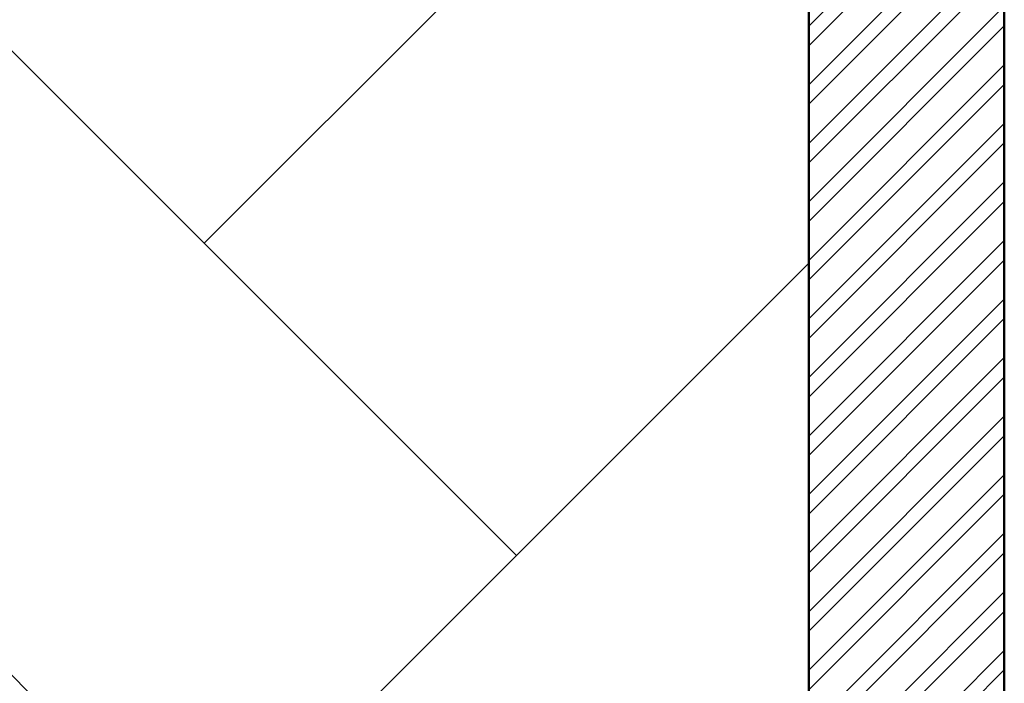
# Model space of a CAD drawing. Units: inches. Extents: x 3590 to 5167, y 65 to 1917.
# Tile 45 of 100: x 5035 to 5080, y 1388 to 1418. Entities that reach past the tile are written whole.
import ezdxf

# ---------------------------------------------------------------- set-up
doc = ezdxf.new("R2010")
doc.units = ezdxf.units.IN
for name, color, linetype, lineweight in [('A-FLOR-PATT', 8, 'Continuous', 13), ('A-WALL', 7, 'Continuous', 50), ('A-WALL-PATT', 251, 'Continuous', 13)]:
    doc.layers.add(name, color=color, linetype=linetype, lineweight=lineweight)

msp = doc.modelspace()

# ---------------------------------------------------------------- hatches: boundary and pattern name
at = {"layer": 'A-FLOR-PATT', "transparency": 33554687}
h = msp.add_hatch(dxfattribs=at)
h.set_pattern_fill('AR-HBONE', color=256, scale=0.2)
h.set_pattern_definition([(45, (-588.972, 0), (0, 28.73682), [60.96, -20.32]), (135, (-574.604, 14.368), (3e-15, 28.73682), [60.96, -20.32])])
h.paths.add_polyline_path([(5071.274, 1796.999), (4933.274, 1796.999), (4933.274, 1753.999), (4962.774, 1753.999, -0.414214), (4928.774, 1719.999), (4933.274, 1718.999), (4933.274, 1334.999), (5071.274, 1334.999)])
h.paths.add_polyline_path([(4951.78, 1521.077), (4951.715, 1521.04), (4951.563, 1520.895)], flags=16)
h.paths.add_polyline_path([(4952.267, 1521.376), (4952.198, 1521.371), (4952.198, 1521.356)], flags=0)
h.paths.add_polyline_path([(4967.051, 1529.728), (4965.231, 1528.694), (4963.411, 1527.714), (4961.756, 1526.851), (4963.589, 1527.449), (4964.036, 1527.478), (4962.975, 1527.249), (4961.76, 1526.852), (4959.792, 1525.834), (4958.005, 1524.895), (4956.24, 1523.93), (4954.504, 1522.919), (4954.129, 1522.682), (4953.361, 1521.997), (4953.366, 1521.998), (4953.605, 1522.064), (4955.106, 1522.761), (4956.921, 1523.434), (4958.678, 1523.915), (4960.358, 1524.2), (4961.945, 1524.286), (4964.171, 1524.108), (4965.958, 1523.309), (4963.863, 1522.976), (4965.187, 1522.499), (4963.366, 1522.497), (4961.545, 1522.487), (4959.764, 1522.461), (4958.304, 1522.419), (4957.974, 1522.388), (4956.307, 1522.232), (4954.718, 1522.071), (4953.251, 1521.899), (4953.525, 1521.623), (4954.331, 1521.379), (4956.243, 1521.23), (4958.039, 1520.93), (4959.684, 1520.483), (4961.16, 1519.896), (4963.107, 1518.8), (4964.393, 1517.325), (4962.973, 1517.726), (4964.558, 1516.661), (4965.407, 1515.708), (4963.507, 1516.322), (4961.68, 1517.005), (4959.935, 1517.745), (4958.282, 1518.528), (4956.732, 1519.343), (4955.295, 1520.175), (4954.672, 1520.572), (4954.513, 1520.627), (4955.658, 1519.318), (4956.703, 1517.982), (4957.644, 1516.647), (4958.485, 1515.334), (4959.55, 1513.524), (4960.438, 1511.769), (4958.841, 1513.62), (4957.452, 1515.325), (4955.819, 1517.459), (4956.665, 1515.448), (4957.111, 1513.923), (4957.447, 1511.714), (4957.076, 1509.793), (4956.538, 1511.11), (4955.992, 1512.569), (4955.444, 1514.125), (4954.898, 1515.735), (4954.357, 1517.356), (4953.824, 1518.943), (4953.305, 1520.452), (4953.065, 1521.116), (4952.971, 1521.146), (4952.949, 1521.086), (4952.73, 1520.199), (4953.37, 1518.024), (4953.757, 1516.373), (4954.051, 1514.765), (4954.264, 1513.221), (4954.471, 1511.131), (4954.497, 1510.402), (4954.409, 1511.76), (4954.264, 1513.221), (4954.051, 1514.765), (4953.757, 1516.373), (4953.37, 1518.024), (4952.877, 1519.698), (4952.716, 1520.141), (4952.533, 1519.059), (4952.374, 1517.789), (4952.219, 1516.312), (4952.046, 1514.6), (4951.833, 1512.626), (4951.557, 1510.363), (4951.203, 1512.168), (4950.852, 1514.339), (4950.985, 1516.376), (4951.66, 1518.286), (4952.593, 1520.481), (4952.357, 1521.13), (4951.855, 1520.328), (4950.839, 1518.908), (4949.777, 1517.587), (4948.916, 1516.617), (4948.111, 1515.256), (4947.089, 1513.554), (4945.889, 1511.615), (4946.326, 1513.402), (4946.562, 1514.249), (4945.528, 1513.327), (4944.581, 1512.531), (4946.018, 1514.508), (4947.204, 1516.048), (4947.893, 1517.313), (4949.307, 1518.764), (4950.414, 1519.767), (4950.451, 1519.806), (4952.267, 1521.376), (4951.645, 1521.493), (4950.404, 1521.18), (4948.044, 1520.359), (4946.119, 1519.452), (4944.572, 1518.475), (4943.35, 1517.443), (4941.997, 1515.92), (4941.661, 1515.275), (4942.813, 1516.99), (4944.572, 1518.475), (4946.119, 1519.452), (4948.044, 1520.359), (4950.404, 1521.18), (4951.645, 1521.493), (4949.647, 1521.868), (4948.6, 1521.756), (4947.126, 1521.57), (4945.42, 1521.348), (4943.45, 1521.105), (4941.183, 1520.856), (4942.86, 1521.613), (4943.873, 1522.03), (4942.952, 1521.909), (4941.41, 1521.485), (4939.543, 1520.67), (4938.968, 1520.226), (4940.733, 1521.299), (4942.952, 1521.909), (4943.702, 1522.008), (4945.894, 1522.7), (4947.565, 1522.714), (4948.921, 1522.566), (4951.131, 1522.183), (4950.971, 1522.297), (4948.129, 1523.006), (4946.035, 1523.707), (4944.232, 1524.521), (4942.707, 1525.461), (4941.444, 1526.537), (4940.43, 1527.761), (4939.649, 1529.143), (4941.421, 1528.122), (4943.147, 1527.132), (4944.841, 1526.175), (4946.514, 1525.25), (4948.179, 1524.359), (4948.365, 1524.263), (4946.475, 1526.045), (4945.181, 1527.54), (4944.19, 1529.033), (4943.496, 1530.54), (4943.278, 1531.36), (4942.498, 1531.919), (4943.114, 1531.762), (4942.959, 1533.659), (4944.14, 1531.989), (4944.612, 1531.323), (4946.202, 1530.463), (4947.486, 1529.509), (4948.79, 1528.226), (4950.368, 1526.237), (4949.485, 1528.155), (4948.851, 1530.123), (4948.491, 1532.041), (4948.381, 1533.918), (4948.501, 1535.76), (4948.827, 1537.573), (4949.418, 1535.565), (4949.957, 1533.569), (4950.464, 1531.586), (4950.961, 1529.617), (4951.391, 1527.954), (4951.724, 1530.687), (4952.201, 1532.58), (4952.889, 1534.33), (4953.77, 1535.951), (4954.827, 1537.46), (4954.521, 1535.39), (4954.273, 1533.937), (4955.58, 1535.663), (4956.748, 1536.739), (4956.159, 1534.78), (4955.589, 1532.873), (4955.043, 1531.006), (4954.525, 1529.166), (4954.038, 1527.341), (4953.638, 1525.733), (4953.611, 1525.586), (4953.398, 1524.166), (4953.382, 1524.009), (4954.07, 1525.476), (4954.912, 1527.022), (4956.136, 1528.894), (4957.847, 1530.577), (4959.376, 1531.54), (4958.256, 1530.104), (4957.143, 1528.663), (4956.066, 1527.243), (4955.056, 1525.871), (4954.141, 1524.571), (4953.352, 1523.372), (4953.311, 1523.303), (4953.273, 1522.925), (4953.261, 1522.382), (4954.103, 1523.373), (4954.63, 1524.284), (4955.961, 1526.358), (4957.23, 1528.13), (4958.421, 1529.609), (4960.037, 1531.368), (4961.374, 1532.375), (4962.101, 1532.77), (4961.07, 1531.061), (4959.987, 1529.438), (4958.869, 1527.908), (4958.15, 1527.007), (4959.803, 1528.003), (4961.589, 1528.793), (4963.391, 1529.328), (4965.211, 1529.632)], flags=16)
h.paths.add_polyline_path([(4962.944, 1523.182), (4961.107, 1523.422), (4960.392, 1523.362), (4962.35, 1523.331)], flags=0)
h.paths.add_polyline_path([(5049.541, 1584.551), (5049.476, 1584.515), (5049.325, 1584.37)], flags=16)
h.paths.add_polyline_path([(5050.028, 1584.851), (5049.959, 1584.845), (5049.959, 1584.83)], flags=0)
h.paths.add_polyline_path([(5042.333, 1581.949), (5043.88, 1582.926), (5045.806, 1583.833), (5048.165, 1584.654), (5049.406, 1584.967), (5047.408, 1585.342), (5046.361, 1585.231), (5044.888, 1585.044), (5043.181, 1584.822), (5041.211, 1584.579), (5038.944, 1584.33), (5040.622, 1585.087), (5041.634, 1585.504), (5040.713, 1585.383), (5039.171, 1584.959), (5037.304, 1584.144), (5036.729, 1583.7), (5038.494, 1584.773), (5040.713, 1585.383), (5041.463, 1585.482), (5043.655, 1586.174), (5045.326, 1586.188), (5046.682, 1586.04), (5048.893, 1585.657), (5048.732, 1585.771), (5045.891, 1586.48), (5043.796, 1587.181), (5041.994, 1587.996), (5040.468, 1588.935), (5039.205, 1590.011), (5038.191, 1591.235), (5037.41, 1592.617), (5039.182, 1591.596), (5040.909, 1590.607), (5042.602, 1589.649), (5044.275, 1588.724), (5045.94, 1587.833), (5046.126, 1587.738), (5044.237, 1589.519), (5042.942, 1591.015), (5041.952, 1592.508), (5041.257, 1594.014), (5041.039, 1594.834), (5040.26, 1595.393), (5040.875, 1595.237), (5040.721, 1597.133), (5041.901, 1595.463), (5042.373, 1594.798), (5043.963, 1593.938), (5045.247, 1592.983), (5046.552, 1591.701), (5048.129, 1589.712), (5047.247, 1591.63), (5046.613, 1593.597), (5046.252, 1595.515), (5046.142, 1597.392), (5046.262, 1599.234), (5046.588, 1601.047), (5047.179, 1599.039), (5047.718, 1597.043), (5048.225, 1595.06), (5048.722, 1593.091), (5049.152, 1591.429), (5049.485, 1594.161), (5049.962, 1596.054), (5050.65, 1597.804), (5051.532, 1599.425), (5052.589, 1600.934), (5052.283, 1598.864), (5052.034, 1597.411), (5053.341, 1599.137), (5054.509, 1600.213), (5053.92, 1598.254), (5053.35, 1596.348), (5052.805, 1594.48), (5052.286, 1592.64), (5051.799, 1590.815), (5051.4, 1589.207), (5051.373, 1589.06), (5051.159, 1587.64), (5051.143, 1587.483), (5051.831, 1588.95), (5052.673, 1590.496), (5053.898, 1592.368), (5055.608, 1594.051), (5057.137, 1595.014), (5056.017, 1593.578), (5054.904, 1592.137), (5053.828, 1590.717), (5052.817, 1589.345), (5051.902, 1588.046), (5051.113, 1586.846), (5051.072, 1586.777), (5051.034, 1586.399), (5051.022, 1585.856), (5051.864, 1586.847), (5052.391, 1587.758), (5053.723, 1589.832), (5054.991, 1591.604), (5056.182, 1593.083), (5057.798, 1594.842), (5059.135, 1595.849), (5059.863, 1596.244), (5058.831, 1594.535), (5057.749, 1592.912), (5056.63, 1591.382), (5055.912, 1590.482), (5057.564, 1591.477), (5059.35, 1592.267), (5061.152, 1592.802), (5062.972, 1593.106), (5064.812, 1593.203), (5062.992, 1592.169), (5061.172, 1591.188), (5059.518, 1590.325), (5061.35, 1590.924), (5061.797, 1590.952), (5060.737, 1590.723), (5059.521, 1590.326), (5057.553, 1589.308), (5055.766, 1588.369), (5054.002, 1587.404), (5052.265, 1586.393), (5051.891, 1586.156), (5051.122, 1585.471), (5051.127, 1585.472), (5051.366, 1585.538), (5052.867, 1586.235), (5054.682, 1586.908), (5056.439, 1587.389), (5058.12, 1587.675), (5059.706, 1587.76), (5061.933, 1587.583), (5063.719, 1586.783), (5061.624, 1586.45), (5062.949, 1585.973), (5061.127, 1585.971), (5059.307, 1585.961), (5057.525, 1585.935), (5056.065, 1585.893), (5055.735, 1585.862), (5054.068, 1585.707), (5052.479, 1585.546), (5051.012, 1585.373), (5051.286, 1585.097), (5052.092, 1584.853), (5054.004, 1584.704), (5055.8, 1584.404), (5057.446, 1583.958), (5058.921, 1583.37), (5060.868, 1582.274), (5062.154, 1580.799), (5060.734, 1581.2), (5062.32, 1580.135), (5063.168, 1579.182), (5061.269, 1579.796), (5059.441, 1580.479), (5057.696, 1581.219), (5056.043, 1582.003), (5054.493, 1582.817), (5053.057, 1583.649), (5052.433, 1584.047), (5052.274, 1584.101), (5053.42, 1582.793), (5054.464, 1581.457), (5055.405, 1580.121), (5056.247, 1578.809), (5057.311, 1576.998), (5058.199, 1575.244), (5056.602, 1577.094), (5055.213, 1578.799), (5053.58, 1580.933), (5054.427, 1578.922), (5054.872, 1577.397), (5055.208, 1575.189), (5054.838, 1573.267), (5054.299, 1574.584), (5053.754, 1576.043), (5053.206, 1577.599), (5052.659, 1579.209), (5052.118, 1580.83), (5051.585, 1582.417), (5051.066, 1583.927), (5050.826, 1584.59), (5050.733, 1584.62), (5050.711, 1584.561), (5050.491, 1583.673), (5051.131, 1581.498), (5051.518, 1579.847), (5051.813, 1578.24), (5052.026, 1576.695), (5052.233, 1574.605), (5052.258, 1573.876), (5052.17, 1575.234), (5052.026, 1576.695), (5051.813, 1578.24), (5051.518, 1579.847), (5051.131, 1581.498), (5050.638, 1583.172), (5050.477, 1583.615), (5050.294, 1582.533), (5050.136, 1581.263), (5049.981, 1579.786), (5049.807, 1578.074), (5049.594, 1576.1), (5049.318, 1573.837), (5048.965, 1575.642), (5048.613, 1577.813), (5048.747, 1579.85), (5049.421, 1581.76), (5050.354, 1583.955), (5050.118, 1584.604), (5049.616, 1583.802), (5048.6, 1582.382), (5047.538, 1581.061), (5046.677, 1580.091), (5045.872, 1578.73), (5044.85, 1577.028), (5043.651, 1575.089), (5044.087, 1576.877), (5044.324, 1577.723), (5043.289, 1576.801), (5042.342, 1576.005), (5043.779, 1577.982), (5044.966, 1579.522), (5045.655, 1580.787), (5047.068, 1582.239), (5048.175, 1583.241), (5048.213, 1583.28), (5050.028, 1584.851), (5049.406, 1584.967), (5048.165, 1584.654), (5045.806, 1583.833), (5043.88, 1582.926), (5042.333, 1581.949), (5041.111, 1580.917), (5039.758, 1579.394), (5039.423, 1578.749), (5040.575, 1580.464)], flags=16)
h.paths.add_polyline_path([(4954.799, 1533.12), (4954.262, 1532.079), (4953.831, 1530.935), (4953.505, 1529.636), (4953.283, 1528.133), (4953.167, 1526.376), (4953.156, 1524.315), (4953.277, 1521.236), (4952.802, 1521.842), (4951.557, 1521.998), (4950.976, 1521.961), (4952.661, 1521.941), (4952.802, 1521.842), (4953.152, 1523.593), (4953.167, 1526.376), (4953.283, 1528.133), (4953.609, 1530.346), (4954.456, 1532.592)], flags=0)
h.paths.add_polyline_path([(5050.563, 1585.316), (5049.318, 1585.472), (5048.737, 1585.435), (5050.422, 1585.415), (5050.563, 1585.316), (5050.914, 1587.067), (5050.928, 1589.851), (5051.045, 1591.607), (5051.371, 1593.82), (5052.217, 1596.066), (5052.56, 1596.594), (5052.024, 1595.554), (5051.592, 1594.409), (5051.266, 1593.11), (5051.045, 1591.607), (5050.928, 1589.851), (5050.918, 1587.789), (5051.038, 1584.71)], flags=0)
h.paths.add_polyline_path([(5058.153, 1586.836), (5060.111, 1586.805), (5060.705, 1586.656), (5058.868, 1586.896)], flags=0)
h.paths.add_polyline_path([(5049.541, 1430.936), (5049.476, 1430.9), (5049.325, 1430.755)], flags=16)
h.paths.add_polyline_path([(5050.028, 1431.236), (5049.959, 1431.231), (5049.959, 1431.215)], flags=0)
h.paths.add_polyline_path([(5046.588, 1447.432), (5047.179, 1445.425), (5047.718, 1443.429), (5048.225, 1441.446), (5048.722, 1439.476), (5049.152, 1437.814), (5049.485, 1440.546), (5049.962, 1442.439), (5050.65, 1444.189), (5051.532, 1445.811), (5052.589, 1447.319), (5052.283, 1445.249), (5052.034, 1443.796), (5053.341, 1445.522), (5054.509, 1446.598), (5053.92, 1444.64), (5053.35, 1442.733), (5052.805, 1440.865), (5052.286, 1439.025), (5051.799, 1437.201), (5051.4, 1435.592), (5051.373, 1435.445), (5051.159, 1434.025), (5051.143, 1433.868), (5051.831, 1435.335), (5052.673, 1436.881), (5053.898, 1438.753), (5055.608, 1440.436), (5057.137, 1441.4), (5056.017, 1439.963), (5054.904, 1438.522), (5053.828, 1437.102), (5052.817, 1435.73), (5051.902, 1434.431), (5051.113, 1433.231), (5051.072, 1433.162), (5051.034, 1432.784), (5051.022, 1432.242), (5051.864, 1433.232), (5052.391, 1434.143), (5053.723, 1436.217), (5054.991, 1437.989), (5056.182, 1439.468), (5057.798, 1441.227), (5059.135, 1442.235), (5059.863, 1442.629), (5058.831, 1440.921), (5057.749, 1439.298), (5056.63, 1437.767), (5055.912, 1436.867), (5057.564, 1437.863), (5059.35, 1438.652), (5061.152, 1439.187), (5062.972, 1439.491), (5064.812, 1439.588), (5062.992, 1438.554), (5061.172, 1437.573), (5059.518, 1436.71), (5061.35, 1437.309), (5061.797, 1437.337), (5060.737, 1437.108), (5059.521, 1436.711), (5057.553, 1435.693), (5055.766, 1434.754), (5054.002, 1433.789), (5052.265, 1432.778), (5051.891, 1432.541), (5051.122, 1431.856), (5051.127, 1431.857), (5051.366, 1431.923), (5052.867, 1432.62), (5054.682, 1433.293), (5056.439, 1433.775), (5058.12, 1434.06), (5059.706, 1434.145), (5061.933, 1433.968), (5063.719, 1433.168), (5061.624, 1432.835), (5062.949, 1432.358), (5061.127, 1432.357), (5059.307, 1432.346), (5057.525, 1432.32), (5056.065, 1432.278), (5055.735, 1432.248), (5054.068, 1432.092), (5052.479, 1431.931), (5051.012, 1431.759), (5051.286, 1431.482), (5052.092, 1431.238), (5054.004, 1431.089), (5055.8, 1430.789), (5057.446, 1430.343), (5058.921, 1429.755), (5060.868, 1428.66), (5062.154, 1427.185), (5060.734, 1427.585), (5062.32, 1426.52), (5063.168, 1425.567), (5061.269, 1426.181), (5059.441, 1426.865), (5057.696, 1427.604), (5056.043, 1428.388), (5054.493, 1429.202), (5053.057, 1430.034), (5052.433, 1430.432), (5052.274, 1430.487), (5053.42, 1429.178), (5054.464, 1427.842), (5055.405, 1426.506), (5056.247, 1425.194), (5057.311, 1423.383), (5058.199, 1421.629), (5056.602, 1423.479), (5055.213, 1425.184), (5053.58, 1427.318), (5054.427, 1425.307), (5054.872, 1423.782), (5055.208, 1421.574), (5054.838, 1419.652), (5054.299, 1420.97), (5053.754, 1422.428), (5053.206, 1423.984), (5052.659, 1425.595), (5052.118, 1427.215), (5051.585, 1428.802), (5051.066, 1430.312), (5050.826, 1430.975), (5050.733, 1431.005), (5050.711, 1430.946), (5050.491, 1430.058), (5051.131, 1427.883), (5051.518, 1426.232), (5051.813, 1424.625), (5052.026, 1423.081), (5052.233, 1420.991), (5052.258, 1420.261), (5052.17, 1421.619), (5052.026, 1423.081), (5051.813, 1424.625), (5051.518, 1426.232), (5051.131, 1427.883), (5050.638, 1429.558), (5050.477, 1430.001), (5050.294, 1428.918), (5050.136, 1427.648), (5049.981, 1426.171), (5049.807, 1424.459), (5049.594, 1422.485), (5049.318, 1420.222), (5048.965, 1422.028), (5048.613, 1424.199), (5048.747, 1426.235), (5049.421, 1428.146), (5050.354, 1430.34), (5050.118, 1430.989), (5049.616, 1430.187), (5048.6, 1428.768), (5047.538, 1427.446), (5046.677, 1426.477), (5045.872, 1425.116), (5044.85, 1423.413), (5043.651, 1421.474), (5044.087, 1423.262), (5044.324, 1424.109), (5043.289, 1423.186), (5042.342, 1422.391), (5043.779, 1424.368), (5044.966, 1425.907), (5045.655, 1427.173), (5047.068, 1428.624), (5048.175, 1429.627), (5048.213, 1429.666), (5050.028, 1431.236), (5049.406, 1431.353), (5048.165, 1431.039), (5045.806, 1430.218), (5043.88, 1429.311), (5042.333, 1428.334), (5041.111, 1427.302), (5039.758, 1425.779), (5039.423, 1425.134), (5040.575, 1426.849), (5042.333, 1428.334), (5043.88, 1429.311), (5045.806, 1430.218), (5048.165, 1431.039), (5049.406, 1431.353), (5047.408, 1431.727), (5046.361, 1431.616), (5044.888, 1431.429), (5043.181, 1431.207), (5041.211, 1430.964), (5038.944, 1430.715), (5040.622, 1431.472), (5041.634, 1431.89), (5040.713, 1431.769), (5039.171, 1431.345), (5037.304, 1430.53), (5036.729, 1430.085), (5038.494, 1431.158), (5040.713, 1431.769), (5041.463, 1431.867), (5043.655, 1432.559), (5045.326, 1432.573), (5046.682, 1432.425), (5048.893, 1432.042), (5048.732, 1432.156), (5045.891, 1432.865), (5043.796, 1433.566), (5041.994, 1434.381), (5040.468, 1435.321), (5039.205, 1436.396), (5038.191, 1437.62), (5037.41, 1439.002), (5039.182, 1437.982), (5040.909, 1436.992), (5042.602, 1436.034), (5044.275, 1435.109), (5045.94, 1434.218), (5046.126, 1434.123), (5044.237, 1435.904), (5042.942, 1437.4), (5041.952, 1438.893), (5041.257, 1440.399), (5041.039, 1441.219), (5040.26, 1441.778), (5040.875, 1441.622), (5040.721, 1443.518), (5041.901, 1441.848), (5042.373, 1441.183), (5043.963, 1440.323), (5045.247, 1439.369), (5046.552, 1438.086), (5048.129, 1436.097), (5047.247, 1438.015), (5046.613, 1439.982), (5046.252, 1441.901), (5046.142, 1443.778), (5046.262, 1445.619)], flags=16)
h.paths.add_polyline_path([(5052.382, 1444.255), (5051.623, 1442.78), (5052.024, 1441.939), (5052.56, 1442.98)], flags=0)
h.paths.add_polyline_path([(5050.563, 1431.701), (5049.318, 1431.857), (5048.737, 1431.821), (5050.422, 1431.8)], flags=0)
h.paths.add_polyline_path([(5058.153, 1433.221), (5060.111, 1433.19), (5060.705, 1433.041), (5058.868, 1433.281)], flags=0)
h.paths.add_polyline_path([(5049.541, 1352.285), (5049.476, 1352.249), (5049.325, 1352.104)], flags=16)
h.paths.add_polyline_path([(5050.028, 1352.585), (5049.959, 1352.58), (5049.959, 1352.564)], flags=0)
h.paths.add_polyline_path([(5046.588, 1368.781), (5047.179, 1366.774), (5047.718, 1364.778), (5048.225, 1362.795), (5048.722, 1360.825), (5049.152, 1359.163), (5049.485, 1361.896), (5049.962, 1363.789), (5050.65, 1365.538), (5051.532, 1367.16), (5052.589, 1368.669), (5052.283, 1366.598), (5052.034, 1365.145), (5053.341, 1366.871), (5054.509, 1367.947), (5053.92, 1365.989), (5053.35, 1364.082), (5052.805, 1362.214), (5052.286, 1360.374), (5051.799, 1358.55), (5051.4, 1356.942), (5051.373, 1356.794), (5051.159, 1355.374), (5051.143, 1355.218), (5051.831, 1356.684), (5052.673, 1358.23), (5053.898, 1360.102), (5055.608, 1361.786), (5057.137, 1362.749), (5056.017, 1361.313), (5054.904, 1359.872), (5053.828, 1358.452), (5052.817, 1357.079), (5051.902, 1355.78), (5051.113, 1354.581), (5051.072, 1354.512), (5051.034, 1354.133), (5051.022, 1353.591), (5051.864, 1354.581), (5052.391, 1355.492), (5053.723, 1357.566), (5054.991, 1359.338), (5056.182, 1360.817), (5057.798, 1362.577), (5059.135, 1363.584), (5059.863, 1363.979), (5058.831, 1362.27), (5057.749, 1360.647), (5056.63, 1359.117), (5055.912, 1358.216), (5057.564, 1359.212), (5059.35, 1360.001), (5061.152, 1360.536), (5062.972, 1360.841), (5064.812, 1360.937), (5062.992, 1359.903), (5061.172, 1358.923), (5059.518, 1358.059), (5061.35, 1358.658), (5061.797, 1358.687), (5060.737, 1358.458), (5059.521, 1358.061), (5057.553, 1357.043), (5055.766, 1356.103), (5054.002, 1355.138), (5052.265, 1354.127), (5051.891, 1353.89), (5051.122, 1353.206), (5051.127, 1353.206), (5051.366, 1353.272), (5052.867, 1353.969), (5054.682, 1354.643), (5056.439, 1355.124), (5058.12, 1355.409), (5059.706, 1355.495), (5061.933, 1355.317), (5063.719, 1354.518), (5061.624, 1354.184), (5062.949, 1353.708), (5061.127, 1353.706), (5059.307, 1353.695), (5057.525, 1353.669), (5056.065, 1353.627), (5055.735, 1353.597), (5054.068, 1353.441), (5052.479, 1353.28), (5051.012, 1353.108), (5051.286, 1352.831), (5052.092, 1352.587), (5054.004, 1352.439), (5055.8, 1352.138), (5057.446, 1351.692), (5058.921, 1351.104), (5060.868, 1350.009), (5062.154, 1348.534), (5060.734, 1348.935), (5062.32, 1347.869), (5063.168, 1346.916), (5061.269, 1347.53), (5059.441, 1348.214), (5057.696, 1348.954), (5056.043, 1349.737), (5054.493, 1350.551), (5053.057, 1351.383), (5052.433, 1351.781), (5052.274, 1351.836), (5053.42, 1350.527), (5054.464, 1349.191), (5055.405, 1347.855), (5056.247, 1346.543), (5057.311, 1344.733), (5058.199, 1342.978), (5056.602, 1344.828), (5055.213, 1346.534), (5053.58, 1348.667), (5054.427, 1346.656), (5054.872, 1345.132), (5055.208, 1342.923), (5054.838, 1341.002), (5054.299, 1342.319), (5053.754, 1343.778), (5053.206, 1345.334), (5052.659, 1346.944), (5052.118, 1348.564), (5051.585, 1350.151), (5051.066, 1351.661), (5050.826, 1352.324), (5050.733, 1352.355), (5050.711, 1352.295), (5050.491, 1351.408), (5051.131, 1349.232), (5051.518, 1347.581), (5051.813, 1345.974), (5052.026, 1344.43), (5052.233, 1342.34), (5052.258, 1341.61), (5052.17, 1342.969), (5052.026, 1344.43), (5051.813, 1345.974), (5051.518, 1347.581), (5051.131, 1349.232), (5050.638, 1350.907), (5050.477, 1351.35), (5050.294, 1350.267), (5050.136, 1348.997), (5049.981, 1347.52), (5049.807, 1345.809), (5049.594, 1343.835), (5049.318, 1341.571), (5048.965, 1343.377), (5048.613, 1345.548), (5048.747, 1347.585), (5049.421, 1349.495), (5050.354, 1351.689), (5050.118, 1352.339), (5049.616, 1351.536), (5048.6, 1350.117), (5047.538, 1348.795), (5046.677, 1347.826), (5045.872, 1346.465), (5044.85, 1344.763), (5043.651, 1342.824), (5044.087, 1344.611), (5044.324, 1345.458), (5043.289, 1344.535), (5042.342, 1343.74), (5043.779, 1345.717), (5044.966, 1347.256), (5045.655, 1348.522), (5047.068, 1349.973), (5048.175, 1350.976), (5048.213, 1351.015), (5050.028, 1352.585), (5049.406, 1352.702), (5048.165, 1352.388), (5045.806, 1351.567), (5043.88, 1350.661), (5042.333, 1349.683), (5041.111, 1348.651), (5039.758, 1347.128), (5039.423, 1346.483), (5040.575, 1348.198), (5042.333, 1349.683), (5043.88, 1350.661), (5045.806, 1351.567), (5048.165, 1352.388), (5049.406, 1352.702), (5047.408, 1353.076), (5046.361, 1352.965), (5044.888, 1352.779), (5043.181, 1352.556), (5041.211, 1352.313), (5038.944, 1352.065), (5040.622, 1352.821), (5041.634, 1353.239), (5040.713, 1353.118), (5039.171, 1352.694), (5037.304, 1351.879), (5036.729, 1351.434), (5038.494, 1352.508), (5040.713, 1353.118), (5041.463, 1353.216), (5043.655, 1353.909), (5045.326, 1353.923), (5046.682, 1353.774), (5048.893, 1353.391), (5048.732, 1353.506), (5045.891, 1354.214), (5043.796, 1354.915), (5041.994, 1355.73), (5040.468, 1356.67), (5039.205, 1357.746), (5038.191, 1358.969), (5037.41, 1360.352), (5039.182, 1359.331), (5040.909, 1358.341), (5042.602, 1357.383), (5044.275, 1356.458), (5045.94, 1355.567), (5046.126, 1355.472), (5044.237, 1357.253), (5042.942, 1358.749), (5041.952, 1360.242), (5041.257, 1361.748), (5041.039, 1362.568), (5040.26, 1363.128), (5040.875, 1362.971), (5040.721, 1364.867), (5041.901, 1363.197), (5042.373, 1362.532), (5043.963, 1361.672), (5045.247, 1360.718), (5046.552, 1359.435), (5048.129, 1357.446), (5047.247, 1359.364), (5046.613, 1361.331), (5046.252, 1363.25), (5046.142, 1365.127), (5046.262, 1366.969)], flags=16)
h.paths.add_polyline_path([(5052.382, 1365.604), (5051.623, 1364.129), (5052.024, 1363.288), (5052.56, 1364.329)], flags=0)
h.paths.add_polyline_path([(4951.78, 1698.041), (4951.715, 1698.005), (4951.563, 1697.859)], flags=16)
h.paths.add_polyline_path([(4952.267, 1698.341), (4952.198, 1698.335), (4952.198, 1698.32)], flags=0)
h.paths.add_polyline_path([(4957.076, 1686.757), (4956.538, 1688.074), (4955.992, 1689.533), (4955.444, 1691.089), (4954.898, 1692.699), (4954.357, 1694.32), (4953.824, 1695.907), (4953.305, 1697.417), (4953.065, 1698.08), (4952.971, 1698.11), (4952.949, 1698.051), (4952.73, 1697.163), (4953.37, 1694.988), (4953.757, 1693.337), (4954.051, 1691.729), (4954.264, 1690.185), (4954.471, 1688.095), (4954.497, 1687.366), (4954.409, 1688.724), (4954.264, 1690.185), (4954.051, 1691.729), (4953.757, 1693.337), (4953.37, 1694.988), (4952.877, 1696.662), (4952.716, 1697.105), (4952.533, 1696.023), (4952.374, 1694.753), (4952.219, 1693.276), (4952.046, 1691.564), (4951.833, 1689.59), (4951.557, 1687.327), (4951.203, 1689.132), (4950.852, 1691.303), (4950.985, 1693.34), (4951.66, 1695.25), (4952.593, 1697.445), (4952.357, 1698.094), (4951.855, 1697.292), (4950.839, 1695.872), (4949.777, 1694.551), (4948.916, 1693.581), (4948.111, 1692.22), (4947.089, 1690.518), (4945.889, 1688.579), (4946.326, 1690.366), (4946.562, 1691.213), (4945.528, 1690.291), (4944.581, 1689.495), (4946.018, 1691.472), (4947.204, 1693.012), (4947.893, 1694.277), (4949.307, 1695.729), (4950.414, 1696.731), (4950.451, 1696.77), (4952.267, 1698.341), (4951.645, 1698.457), (4950.404, 1698.144), (4948.044, 1697.323), (4946.119, 1696.416), (4944.572, 1695.439), (4943.35, 1694.407), (4941.997, 1692.884), (4941.661, 1692.239), (4942.813, 1693.954), (4944.572, 1695.439), (4946.119, 1696.416), (4948.044, 1697.323), (4950.404, 1698.144), (4951.645, 1698.457), (4949.647, 1698.832), (4948.6, 1698.72), (4947.126, 1698.534), (4945.42, 1698.312), (4943.45, 1698.069), (4941.183, 1697.82), (4942.86, 1698.577), (4943.873, 1698.994), (4942.952, 1698.873), (4941.41, 1698.449), (4939.543, 1697.634), (4938.968, 1697.19), (4940.733, 1698.263), (4942.952, 1698.873), (4943.702, 1698.972), (4945.894, 1699.664), (4947.565, 1699.678), (4948.921, 1699.53), (4951.131, 1699.147), (4950.971, 1699.261), (4948.129, 1699.97), (4946.035, 1700.671), (4944.232, 1701.486), (4942.707, 1702.425), (4941.444, 1703.501), (4940.43, 1704.725), (4939.649, 1706.107), (4941.421, 1705.086), (4943.147, 1704.097), (4944.841, 1703.139), (4946.514, 1702.214), (4948.179, 1701.323), (4948.365, 1701.227), (4946.475, 1703.009), (4945.181, 1704.505), (4944.19, 1705.997), (4943.496, 1707.504), (4943.278, 1708.324), (4942.498, 1708.883), (4943.114, 1708.727), (4942.959, 1710.623), (4944.14, 1708.953), (4944.612, 1708.287), (4946.202, 1707.428), (4947.486, 1706.473), (4948.79, 1705.191), (4950.368, 1703.202), (4949.485, 1705.12), (4948.851, 1707.087), (4948.491, 1709.005), (4948.381, 1710.882), (4948.501, 1712.724), (4948.827, 1714.537), (4949.418, 1712.529), (4949.957, 1710.533), (4950.464, 1708.55), (4950.961, 1706.581), (4951.391, 1704.919), (4951.724, 1707.651), (4952.201, 1709.544), (4952.889, 1711.294), (4953.77, 1712.915), (4954.827, 1714.424), (4954.521, 1712.354), (4954.273, 1710.901), (4955.58, 1712.627), (4956.748, 1713.703), (4956.159, 1711.744), (4955.589, 1709.837), (4955.043, 1707.97), (4954.525, 1706.13), (4954.038, 1704.305), (4953.638, 1702.697), (4953.611, 1702.55), (4953.398, 1701.13), (4953.382, 1700.973), (4954.07, 1702.44), (4954.912, 1703.986), (4956.136, 1705.858), (4957.847, 1707.541), (4959.376, 1708.504), (4958.256, 1707.068), (4957.143, 1705.627), (4956.066, 1704.207), (4955.056, 1702.835), (4954.141, 1701.536), (4953.352, 1700.336), (4953.311, 1700.267), (4953.273, 1699.889), (4953.261, 1699.346), (4954.103, 1700.337), (4954.63, 1701.248), (4955.961, 1703.322), (4957.23, 1705.094), (4958.421, 1706.573), (4960.037, 1708.332), (4961.374, 1709.339), (4962.101, 1709.734), (4961.07, 1708.025), (4959.987, 1706.402), (4958.869, 1704.872), (4958.15, 1703.972), (4959.803, 1704.967), (4961.589, 1705.757), (4963.391, 1706.292), (4965.211, 1706.596), (4967.051, 1706.692), (4965.231, 1705.659), (4963.411, 1704.678), (4961.756, 1703.815), (4963.589, 1704.413), (4964.036, 1704.442), (4962.975, 1704.213), (4961.76, 1703.816), (4959.792, 1702.798), (4958.005, 1701.859), (4956.24, 1700.894), (4954.504, 1699.883), (4954.129, 1699.646), (4953.361, 1698.961), (4953.366, 1698.962), (4953.605, 1699.028), (4955.106, 1699.725), (4956.921, 1700.398), (4958.678, 1700.879), (4960.358, 1701.164), (4961.945, 1701.25), (4964.171, 1701.073), (4965.958, 1700.273), (4963.863, 1699.94), (4965.187, 1699.463), (4963.366, 1699.461), (4961.545, 1699.451), (4959.764, 1699.425), (4958.304, 1699.383), (4957.974, 1699.352), (4956.307, 1699.197), (4954.718, 1699.036), (4953.251, 1698.863), (4953.525, 1698.587), (4954.331, 1698.343), (4956.243, 1698.194), (4958.039, 1697.894), (4959.684, 1697.447), (4961.16, 1696.86), (4963.107, 1695.764), (4964.393, 1694.289), (4962.973, 1694.69), (4964.558, 1693.625), (4965.407, 1692.672), (4963.507, 1693.286), (4961.68, 1693.969), (4959.935, 1694.709), (4958.282, 1695.492), (4956.732, 1696.307), (4955.295, 1697.139), (4954.672, 1697.536), (4954.513, 1697.591), (4955.658, 1696.282), (4956.703, 1694.946), (4957.644, 1693.611), (4958.485, 1692.298), (4959.55, 1690.488), (4960.438, 1688.733), (4958.841, 1690.584), (4957.452, 1692.289), (4955.819, 1694.423), (4956.665, 1692.412), (4957.111, 1690.887), (4957.447, 1688.678)], flags=16)
h.paths.add_polyline_path([(5050.563, 1353.05), (5049.318, 1353.207), (5048.737, 1353.17), (5050.422, 1353.15)], flags=0)
h.paths.add_polyline_path([(4951.78, 1351.486), (4951.715, 1351.45), (4951.563, 1351.305)], flags=16)
h.paths.add_polyline_path([(4952.267, 1351.786), (4952.198, 1351.78), (4952.198, 1351.765)], flags=0)
h.paths.add_polyline_path([(4954.827, 1367.869), (4954.521, 1365.799), (4954.273, 1364.346), (4955.58, 1366.072), (4956.748, 1367.148), (4956.159, 1365.19), (4955.589, 1363.283), (4955.043, 1361.415), (4954.525, 1359.575), (4954.038, 1357.751), (4953.638, 1356.142), (4953.611, 1355.995), (4953.398, 1354.575), (4953.382, 1354.418), (4954.07, 1355.885), (4954.912, 1357.431), (4956.136, 1359.303), (4957.847, 1360.986), (4959.376, 1361.95), (4958.256, 1360.513), (4957.143, 1359.072), (4956.066, 1357.652), (4955.056, 1356.28), (4954.141, 1354.981), (4953.352, 1353.781), (4953.311, 1353.712), (4953.273, 1353.334), (4953.261, 1352.792), (4954.103, 1353.782), (4954.63, 1354.693), (4955.961, 1356.767), (4957.23, 1358.539), (4958.421, 1360.018), (4960.037, 1361.777), (4961.374, 1362.785), (4962.101, 1363.179), (4961.07, 1361.471), (4959.987, 1359.848), (4958.869, 1358.317), (4958.15, 1357.417), (4959.803, 1358.413), (4961.589, 1359.202), (4963.391, 1359.737), (4965.211, 1360.041), (4967.051, 1360.138), (4965.231, 1359.104), (4963.411, 1358.123), (4961.756, 1357.26), (4963.589, 1357.859), (4964.036, 1357.887), (4962.975, 1357.658), (4961.76, 1357.261), (4959.792, 1356.243), (4958.005, 1355.304), (4956.24, 1354.339), (4954.504, 1353.328), (4954.129, 1353.091), (4953.361, 1352.406), (4953.366, 1352.407), (4953.605, 1352.473), (4955.106, 1353.17), (4956.921, 1353.843), (4958.678, 1354.325), (4960.358, 1354.61), (4961.945, 1354.695), (4964.171, 1354.518), (4965.958, 1353.718), (4963.863, 1353.385), (4965.187, 1352.908), (4963.366, 1352.907), (4961.545, 1352.896), (4959.764, 1352.87), (4958.304, 1352.828), (4957.974, 1352.798), (4956.307, 1352.642), (4954.718, 1352.481), (4953.251, 1352.309), (4953.525, 1352.032), (4954.331, 1351.788), (4956.243, 1351.639), (4958.039, 1351.339), (4959.684, 1350.893), (4961.16, 1350.305), (4963.107, 1349.21), (4964.393, 1347.735), (4962.973, 1348.135), (4964.558, 1347.07), (4965.407, 1346.117), (4963.507, 1346.731), (4961.68, 1347.414), (4959.935, 1348.154), (4958.282, 1348.938), (4956.732, 1349.752), (4955.295, 1350.584), (4954.672, 1350.982), (4954.513, 1351.036), (4955.658, 1349.728), (4956.703, 1348.392), (4957.644, 1347.056), (4958.485, 1345.744), (4959.55, 1343.933), (4960.438, 1342.179), (4958.841, 1344.029), (4957.452, 1345.734), (4955.819, 1347.868), (4956.665, 1345.857), (4957.111, 1344.332), (4957.447, 1342.124), (4957.076, 1340.202), (4956.538, 1341.52), (4955.992, 1342.978), (4955.444, 1344.534), (4954.898, 1346.145), (4954.357, 1347.765), (4953.824, 1349.352), (4953.305, 1350.862), (4953.065, 1351.525), (4952.971, 1351.555), (4952.949, 1351.496), (4952.73, 1350.608), (4953.37, 1348.433), (4953.757, 1346.782), (4954.051, 1345.175), (4954.264, 1343.631), (4954.471, 1341.541), (4954.497, 1340.811), (4954.409, 1342.169), (4954.264, 1343.631), (4954.051, 1345.175), (4953.757, 1346.782), (4953.37, 1348.433), (4952.877, 1350.108), (4952.716, 1350.551), (4952.533, 1349.468), (4952.374, 1348.198), (4952.219, 1346.721), (4952.046, 1345.009), (4951.833, 1343.035), (4951.557, 1340.772), (4951.203, 1342.578), (4950.852, 1344.749), (4950.985, 1346.785), (4951.66, 1348.696), (4952.593, 1350.89), (4952.357, 1351.539), (4951.855, 1350.737), (4950.839, 1349.318), (4949.777, 1347.996), (4948.916, 1347.027), (4948.111, 1345.665), (4947.089, 1343.963), (4945.889, 1342.024), (4946.326, 1343.812), (4946.562, 1344.659), (4945.528, 1343.736), (4944.581, 1342.941), (4946.018, 1344.918), (4947.204, 1346.457), (4947.893, 1347.723), (4949.307, 1349.174), (4950.414, 1350.177), (4950.451, 1350.216), (4952.267, 1351.786), (4951.645, 1351.903), (4950.404, 1351.589), (4948.044, 1350.768), (4946.119, 1349.861), (4944.572, 1348.884), (4943.35, 1347.852), (4941.997, 1346.329), (4941.661, 1345.684), (4942.813, 1347.399), (4944.572, 1348.884), (4946.119, 1349.861), (4948.044, 1350.768), (4950.404, 1351.589), (4951.645, 1351.903), (4949.647, 1352.277), (4948.6, 1352.166), (4947.126, 1351.979), (4945.42, 1351.757), (4943.45, 1351.514), (4941.183, 1351.265), (4942.86, 1352.022), (4943.873, 1352.44), (4942.952, 1352.319), (4941.41, 1351.895), (4939.543, 1351.08), (4938.968, 1350.635), (4940.733, 1351.708), (4942.952, 1352.319), (4943.702, 1352.417), (4945.894, 1353.109), (4947.565, 1353.123), (4948.921, 1352.975), (4951.131, 1352.592), (4950.971, 1352.706), (4948.129, 1353.415), (4946.035, 1354.116), (4944.232, 1354.931), (4942.707, 1355.871), (4941.444, 1356.946), (4940.43, 1358.17), (4939.649, 1359.552), (4941.421, 1358.532), (4943.147, 1357.542), (4944.841, 1356.584), (4946.514, 1355.659), (4948.179, 1354.768), (4948.365, 1354.673), (4946.475, 1356.454), (4945.181, 1357.95), (4944.19, 1359.443), (4943.496, 1360.949), (4943.278, 1361.769), (4942.498, 1362.328), (4943.114, 1362.172), (4942.959, 1364.068), (4944.14, 1362.398), (4944.612, 1361.733), (4946.202, 1360.873), (4947.486, 1359.919), (4948.79, 1358.636), (4950.368, 1356.647), (4949.485, 1358.565), (4948.851, 1360.532), (4948.491, 1362.451), (4948.381, 1364.328), (4948.501, 1366.169), (4948.827, 1367.982), (4949.418, 1365.975), (4949.957, 1363.979), (4950.464, 1361.995), (4950.961, 1360.026), (4951.391, 1358.364), (4951.724, 1361.096), (4952.201, 1362.989), (4952.889, 1364.739), (4953.77, 1366.361)], flags=16)
h.paths.add_polyline_path([(4954.799, 1363.53), (4954.262, 1362.489), (4953.831, 1361.344), (4953.505, 1360.045), (4953.283, 1358.543), (4953.167, 1356.786), (4953.156, 1354.724), (4953.277, 1351.646), (4952.802, 1352.251), (4951.557, 1352.407), (4950.976, 1352.371), (4952.661, 1352.35), (4952.802, 1352.251), (4953.152, 1354.002), (4953.167, 1356.786), (4953.283, 1358.543), (4953.609, 1360.755), (4954.456, 1363.001)], flags=0)
h.paths.add_polyline_path([(4952.802, 1698.806), (4951.557, 1698.962), (4950.976, 1698.925), (4952.661, 1698.905), (4952.802, 1698.806), (4953.152, 1700.557), (4953.167, 1703.34), (4953.283, 1705.097), (4953.609, 1707.31), (4954.456, 1709.556), (4954.799, 1710.084), (4954.262, 1709.043), (4953.831, 1707.899), (4953.505, 1706.6), (4953.283, 1705.097), (4953.167, 1703.34), (4953.156, 1701.279), (4953.277, 1698.2)], flags=0)
h.paths.add_polyline_path([(4962.944, 1700.146), (4961.107, 1700.386), (4960.392, 1700.326), (4962.35, 1700.295)], flags=0)
h.paths.add_polyline_path([(5058.153, 1354.57), (5060.111, 1354.539), (5060.705, 1354.391), (5058.868, 1354.631)], flags=0)
h.paths.add_polyline_path([(4962.944, 1353.591), (4961.107, 1353.831), (4960.392, 1353.771), (4962.35, 1353.74)], flags=0)
h.paths.add_polyline_path([(5049.541, 1778.72), (5049.476, 1778.684), (5049.325, 1778.539)], flags=16)
h.paths.add_polyline_path([(5050.028, 1779.02), (5049.959, 1779.014), (5049.959, 1778.999)], flags=0)
h.paths.add_polyline_path([(5052.258, 1768.045), (5052.17, 1769.403), (5052.026, 1770.864), (5051.813, 1772.409), (5051.518, 1774.016), (5051.131, 1775.667), (5050.638, 1777.341), (5050.477, 1777.784), (5050.294, 1776.702), (5050.136, 1775.432), (5049.981, 1773.955), (5049.807, 1772.243), (5049.594, 1770.269), (5049.318, 1768.006), (5048.965, 1769.811), (5048.613, 1771.982), (5048.747, 1774.019), (5049.421, 1775.929), (5050.354, 1778.124), (5050.118, 1778.773), (5049.616, 1777.971), (5048.6, 1776.551), (5047.538, 1775.23), (5046.677, 1774.26), (5045.872, 1772.899), (5044.85, 1771.197), (5043.651, 1769.258), (5044.087, 1771.046), (5044.324, 1771.892), (5043.289, 1770.97), (5042.342, 1770.174), (5043.779, 1772.151), (5044.966, 1773.691), (5045.655, 1774.956), (5047.068, 1776.408), (5048.175, 1777.41), (5048.213, 1777.449), (5050.028, 1779.02), (5049.406, 1779.136), (5048.165, 1778.823), (5045.806, 1778.002), (5043.88, 1777.095), (5042.333, 1776.118), (5041.111, 1775.086), (5039.758, 1773.563), (5039.423, 1772.918), (5040.575, 1774.633), (5042.333, 1776.118), (5043.88, 1777.095), (5045.806, 1778.002), (5048.165, 1778.823), (5049.406, 1779.136), (5047.408, 1779.511), (5046.361, 1779.4), (5044.888, 1779.213), (5043.181, 1778.991), (5041.211, 1778.748), (5038.944, 1778.499), (5040.622, 1779.256), (5041.634, 1779.673), (5040.713, 1779.552), (5039.171, 1779.128), (5037.304, 1778.313), (5036.729, 1777.869), (5038.494, 1778.942), (5040.713, 1779.552), (5041.463, 1779.651), (5043.655, 1780.343), (5045.326, 1780.357), (5046.682, 1780.209), (5048.893, 1779.826), (5048.732, 1779.94), (5045.891, 1780.649), (5043.796, 1781.35), (5041.994, 1782.165), (5040.468, 1783.104), (5039.205, 1784.18), (5038.191, 1785.404), (5037.41, 1786.786), (5039.182, 1785.765), (5040.909, 1784.776), (5042.602, 1783.818), (5044.275, 1782.893), (5045.94, 1782.002), (5046.126, 1781.907), (5044.237, 1783.688), (5042.942, 1785.184), (5041.952, 1786.677), (5041.257, 1788.183), (5041.039, 1789.003), (5040.26, 1789.562), (5040.875, 1789.406), (5040.721, 1791.302), (5041.901, 1789.632), (5042.373, 1788.967), (5043.963, 1788.107), (5045.247, 1787.152), (5046.552, 1785.87), (5048.129, 1783.881), (5047.247, 1785.799), (5046.613, 1787.766), (5046.252, 1789.684), (5046.142, 1791.561), (5046.262, 1793.403), (5046.588, 1795.216), (5047.179, 1793.208), (5047.718, 1791.213), (5048.225, 1789.229), (5048.722, 1787.26), (5049.152, 1785.598), (5049.485, 1788.33), (5049.962, 1790.223), (5050.65, 1791.973), (5051.532, 1793.594), (5052.589, 1795.103), (5052.283, 1793.033), (5052.034, 1791.58), (5053.341, 1793.306), (5054.509, 1794.382), (5053.92, 1792.423), (5053.35, 1790.517), (5052.805, 1788.649), (5052.286, 1786.809), (5051.799, 1784.984), (5051.4, 1783.376), (5051.373, 1783.229), (5051.159, 1781.809), (5051.143, 1781.652), (5051.831, 1783.119), (5052.673, 1784.665), (5053.898, 1786.537), (5055.608, 1788.22), (5057.137, 1789.183), (5056.017, 1787.747), (5054.904, 1786.306), (5053.828, 1784.886), (5052.817, 1783.514), (5051.902, 1782.215), (5051.113, 1781.015), (5051.072, 1780.946), (5051.034, 1780.568), (5051.022, 1780.025), (5051.864, 1781.016), (5052.391, 1781.927), (5053.723, 1784.001), (5054.991, 1785.773), (5056.182, 1787.252), (5057.798, 1789.011), (5059.135, 1790.018), (5059.863, 1790.413), (5058.831, 1788.704), (5057.749, 1787.081), (5056.63, 1785.551), (5055.912, 1784.651), (5057.564, 1785.646), (5059.35, 1786.436), (5061.152, 1786.971), (5062.972, 1787.275), (5064.812, 1787.372), (5062.992, 1786.338), (5061.172, 1785.357), (5059.518, 1784.494), (5061.35, 1785.093), (5061.797, 1785.121), (5060.737, 1784.892), (5059.521, 1784.495), (5057.553, 1783.477), (5055.766, 1782.538), (5054.002, 1781.573), (5052.265, 1780.562), (5051.891, 1780.325), (5051.122, 1779.64), (5051.127, 1779.641), (5051.366, 1779.707), (5052.867, 1780.404), (5054.682, 1781.077), (5056.439, 1781.558), (5058.12, 1781.844), (5059.706, 1781.929), (5061.933, 1781.752), (5063.719, 1780.952), (5061.624, 1780.619), (5062.949, 1780.142), (5061.127, 1780.14), (5059.307, 1780.13), (5057.525, 1780.104), (5056.065, 1780.062), (5055.735, 1780.031), (5054.068, 1779.876), (5052.479, 1779.715), (5051.012, 1779.542), (5051.286, 1779.266), (5052.092, 1779.022), (5054.004, 1778.873), (5055.8, 1778.573), (5057.446, 1778.127), (5058.921, 1777.539), (5060.868, 1776.443), (5062.154, 1774.968), (5060.734, 1775.369), (5062.32, 1774.304), (5063.168, 1773.351), (5061.269, 1773.965), (5059.441, 1774.648), (5057.696, 1775.388), (5056.043, 1776.172), (5054.493, 1776.986), (5053.057, 1777.818), (5052.433, 1778.216), (5052.274, 1778.27), (5053.42, 1776.962), (5054.464, 1775.626), (5055.405, 1774.29), (5056.247, 1772.978), (5057.311, 1771.167), (5058.199, 1769.413), (5056.602, 1771.263), (5055.213, 1772.968), (5053.58, 1775.102), (5054.427, 1773.091), (5054.872, 1771.566), (5055.208, 1769.358), (5054.838, 1767.436), (5054.299, 1768.753), (5053.754, 1770.212), (5053.206, 1771.768), (5052.659, 1773.378), (5052.118, 1774.999), (5051.585, 1776.586), (5051.066, 1778.096), (5050.826, 1778.759), (5050.733, 1778.789), (5050.711, 1778.73), (5050.491, 1777.842), (5051.131, 1775.667), (5051.518, 1774.016), (5051.813, 1772.409), (5052.026, 1770.864), (5052.233, 1768.774)], flags=16)
h.paths.add_polyline_path([(5050.563, 1779.485), (5049.318, 1779.641), (5048.737, 1779.604), (5050.422, 1779.584), (5050.563, 1779.485), (5050.914, 1781.236), (5050.928, 1784.02), (5051.045, 1785.776), (5051.371, 1787.989), (5052.217, 1790.235), (5052.56, 1790.763), (5052.024, 1789.723), (5051.592, 1788.578), (5051.266, 1787.279), (5051.045, 1785.776), (5050.928, 1784.02), (5050.918, 1781.958), (5051.038, 1778.879)], flags=0)
h.paths.add_polyline_path([(5058.153, 1781.005), (5060.111, 1780.974), (5060.705, 1780.825), (5058.868, 1781.065)], flags=0)
at = {"layer": 'A-WALL-PATT', "transparency": 33554687}
h = msp.add_hatch(dxfattribs=at)
h.set_pattern_fill('ANSI32', color=256, scale=0.2)
h.paths.add_polyline_path([(4684.274, 1805.999), (4591.274, 1805.999), (4591.274, 1796.999), (4639.274, 1796.999), (4639.274, 1790.999), (4648.274, 1790.999), (4648.274, 1796.999), (4684.274, 1796.999)])
h.paths.add_polyline_path([(4543.274, 1805.999), (4420.274, 1805.999), (4420.274, 1784.999), (4429.274, 1784.999), (4429.274, 1796.999), (4445.919, 1796.999), (4543.274, 1796.999)])
h.paths.add_polyline_path([(4828.274, 1805.999), (4744.274, 1805.999), (4744.274, 1796.999), (4828.274, 1796.999)])
h.paths.add_polyline_path([(4648.274, 1754.999), (4639.274, 1754.999), (4639.274, 1655.999), (4546.274, 1655.999), (4546.274, 1649.999), (4549.274, 1649.999), (4549.274, 1553.999), (4429.274, 1553.999), (4429.274, 1583.999), (4420.274, 1583.999), (4420.274, 1538.999), (4429.274, 1538.999), (4429.274, 1544.999), (4639.274, 1544.999), (4639.274, 1538.999), (4648.274, 1538.999), (4648.274, 1559.999), (4639.274, 1559.999), (4639.274, 1553.999), (4555.274, 1553.999), (4555.274, 1649.999), (4639.274, 1649.999), (4639.274, 1589.999), (4648.274, 1589.999)])
h.paths.add_polyline_path([(4516.274, 1655.999), (4429.274, 1655.999), (4429.274, 1736.999), (4420.274, 1736.999), (4420.274, 1619.999), (4429.274, 1619.999), (4429.274, 1649.999), (4516.274, 1649.999)], flags=17)
h.paths.add_polyline_path([(5080.274, 1805.999), (4888.274, 1805.999), (4888.274, 1796.999), (4924.274, 1796.999), (4924.274, 1754.999), (4933.274, 1754.999), (4933.274, 1796.999), (5071.274, 1796.999), (5071.274, 1334.999), (4933.274, 1334.999), (4933.274, 1565.999), (4924.274, 1565.999), (4924.274, 1334.999), (4898.774, 1334.999), (4898.774, 1325.999), (5080.274, 1325.999)])
h.paths.add_polyline_path([(4933.274, 1718.999), (4924.274, 1718.999), (4924.274, 1637.999), (4933.274, 1637.999)], flags=17)
h.paths.add_polyline_path([(4802.774, 1334.999), (4777.274, 1334.999), (4777.274, 1502.999), (4756.274, 1502.999), (4756.274, 1493.999), (4768.274, 1493.999), (4768.274, 1430.999), (4696.274, 1430.999), (4696.274, 1493.999), (4708.274, 1493.999), (4708.274, 1502.999), (4639.274, 1502.999), (4639.274, 1493.999), (4687.274, 1493.999), (4687.274, 1430.999), (4681.274, 1430.999), (4681.274, 1421.999), (4768.274, 1421.999), (4768.274, 1334.999), (4726.274, 1334.999), (4726.274, 1325.999), (4802.774, 1325.999)])
h.paths.add_polyline_path([(4690.274, 1334.999), (4648.274, 1334.999), (4648.274, 1352.867), (4648.274, 1421.999), (4651.274, 1421.999), (4651.274, 1430.999), (4639.274, 1430.999), (4639.274, 1334.999), (4633.274, 1334.999), (4633.274, 1325.999), (4690.274, 1325.999)])
h.paths.add_polyline_path([(4585.274, 1334.999), (4584.724, 1334.999), (4429.274, 1334.999), (4429.274, 1490.999), (4420.274, 1490.999), (4420.274, 1325.999), (4585.274, 1325.999)])

# ---------------------------------------------------------------- linework, layer by layer
at = {"layer": 'A-WALL'}
msp.add_line((5071.274, 1334.999), (5071.274, 1796.999), dxfattribs=at)
msp.add_lwpolyline([(5080.274, 1805.999), (5080.274, 1325.999), (4420.274, 1325.999), (4420.274, 1805.999)], close=True, dxfattribs=at)

doc.saveas('drawing.dxf')
